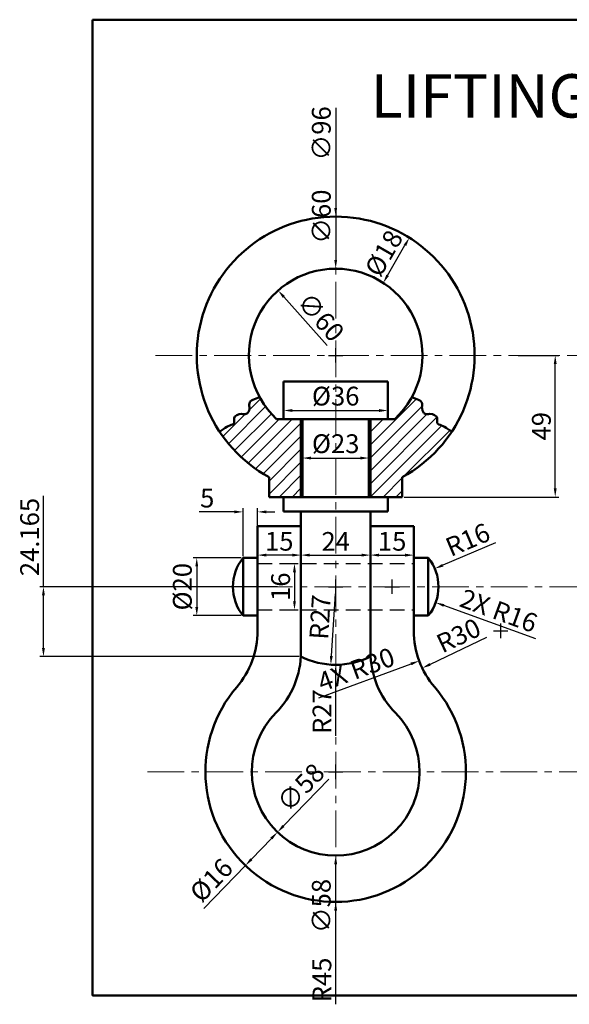
# Model space of a CAD drawing. Units: millimetres. Extents: x 309 to 670, y -17 to 339.
# Tile 1 of 2: x 309 to 498, y -2 to 339. Entities that reach past the tile are written whole.
import ezdxf

# ---------------------------------------------------------------- set-up
doc = ezdxf.new("R2010")
doc.units = ezdxf.units.MM
doc.header["$LTSCALE"] = 0.4
doc.linetypes.add('CENTER', pattern=[50.8, 31.75, -6.35, 6.35, -6.35])
doc.linetypes.add('DASHED', pattern=[19.05, 12.7, -6.35])
for name, color, linetype, lineweight in [('M-CNTR', 1, 'CENTER', 18), ('M-DIMS', 2, 'Continuous', 25), ('M-HATC', 8, 'Continuous', 18), ('M-HIDN', 3, 'DASHED', 25), ('M-OUTL', 7, 'Continuous', 50), ('M-TEXT', 7, 'Continuous', 25), ('M-TTLB', 7, 'Continuous', 50)]:
    doc.layers.add(name, color=color, linetype=linetype, lineweight=lineweight)
doc.styles.get("Standard").update_dxf_attribs({"font": 'arial.ttf'})
doc.dimstyles.new('ISO-25', dxfattribs={"dimtxt": 6.5, "dimasz": 3, "dimexe": 1.25, "dimexo": 0.625, "dimtad": 1, "dimdec": 0, "dimtxsty": 'Standard', "dimcen": 2.5, "dimadec": 0, "dimazin": 0, "dimtfac": 1, "dimtdec": 0, "dimtofl": 0, "dimtmove": 0, "dimatfit": 3, "dimfxl": 1, "dimarcsym": 0})

# ---------------------------------------------------------------- blocks, each defined once
blk = doc.blocks.new('*D13')
at = {"layer": 'Defpoints', "color": 0, "ltscale": 0.4, "transparency": 16777216}
for p in [(437.86, 99.54), (397.62, 57.77)]:
    blk.add_point(p, dxfattribs=at)
at = {"layer": 'M-DIMS', "color": 0, "lineweight": -2, "ltscale": 0.4, "transparency": 16777216}
blk.add_line((415.34, 76.16), (399.7, 59.93), dxfattribs=at)
at = {"layer": 'M-DIMS', "color": 0, "ltscale": 0.4, "transparency": 16777216}
blk.add_solid([(399.34, 60.27), (400.07, 59.58), (397.62, 57.77)], dxfattribs=at)
at = {"layer": 'M-DIMS', "color": 0, "ltscale": 0.4, "transparency": 16777216, "insert": (406.25, 72.67), "char_height": 6.5, "attachment_point": 5, "rotation": 46.0797}
blk.add_mtext('∅58', dxfattribs=at)
blk = doc.blocks.new('*D14')
at = {"layer": 'Defpoints', "color": 0, "ltscale": 0.4, "transparency": 16777216}
for p in [(397.62, 57.77), (386.53, 46.24), (386.53, 46.24)]:
    blk.add_point(p, dxfattribs=at)
at = {"layer": 'M-DIMS', "color": 0, "lineweight": -2, "ltscale": 0.4, "transparency": 16777216}
for p, q in [((397.17, 58.2), (396.72, 58.63)), ((395.54, 55.61), (388.61, 48.4)), ((386.53, 46.24), (372.22, 31.38)), ((386.08, 46.68), (385.63, 47.11))]:
    blk.add_line(p, q, dxfattribs=at)
at = {"layer": 'M-DIMS', "color": 0, "ltscale": 0.4, "transparency": 16777216}
for points in [[(395.18, 55.95), (395.9, 55.26), (397.62, 57.77)], [(388.25, 48.75), (388.97, 48.06), (386.53, 46.24)]]:
    blk.add_solid(points, dxfattribs=at)
at = {"layer": 'M-DIMS', "color": 0, "ltscale": 0.4, "transparency": 16777216, "insert": (375.36, 40.59), "char_height": 6.5, "attachment_point": 5, "rotation": 46.0797}
blk.add_mtext('%%C16', dxfattribs=at)
blk = doc.blocks.new('*D15')
at = {"layer": 'Defpoints', "color": 0, "ltscale": 0.4, "transparency": 16777216}
for p in [(390.74, 168.54), (385.74, 152.66), (390.74, 152.66)]:
    blk.add_point(p, dxfattribs=at)
at = {"layer": 'M-DIMS', "color": 0, "lineweight": -2, "ltscale": 0.4, "transparency": 16777216}
for p, q in [((382.74, 168.54), (370.57, 168.54)), ((385.74, 153.28), (385.74, 169.79)), ((390.74, 153.28), (390.74, 169.79)), ((393.74, 168.54), (396.74, 168.54))]:
    blk.add_line(p, q, dxfattribs=at)
at = {"layer": 'M-DIMS', "color": 0, "ltscale": 0.4, "transparency": 16777216}
for points in [[(382.74, 169.04), (382.74, 168.04), (385.74, 168.54)], [(393.74, 169.04), (393.74, 168.04), (390.74, 168.54)]]:
    blk.add_solid(points, dxfattribs=at)
at = {"layer": 'M-DIMS', "color": 0, "ltscale": 0.4, "transparency": 16777216, "insert": (373.35, 172.47), "char_height": 6.5, "attachment_point": 5}
blk.add_mtext('5', dxfattribs=at)
blk = doc.blocks.new('*D16')
at = {"layer": 'Defpoints', "color": 0, "ltscale": 0.4, "transparency": 16777216}
for p in [(429.74, 157.6), (444.74, 157.6), (444.74, 153.59)]:
    blk.add_point(p, dxfattribs=at)
at = {"layer": 'M-DIMS', "color": 0, "lineweight": -2, "ltscale": 0.4, "transparency": 16777216}
for p, q in [((429.74, 156.97), (429.74, 152.34)), ((444.74, 156.97), (444.74, 152.34)), ((432.74, 153.59), (441.74, 153.59))]:
    blk.add_line(p, q, dxfattribs=at)
at = {"layer": 'M-DIMS', "color": 0, "ltscale": 0.4, "transparency": 16777216}
for points in [[(432.74, 154.09), (432.74, 153.09), (429.74, 153.59)], [(441.74, 154.09), (441.74, 153.09), (444.74, 153.59)]]:
    blk.add_solid(points, dxfattribs=at)
at = {"layer": 'M-DIMS', "color": 0, "ltscale": 0.4, "transparency": 16777216, "insert": (437.24, 157.54), "char_height": 6.5, "attachment_point": 5}
blk.add_mtext('15', dxfattribs=at)
blk = doc.blocks.new('*D17')
at = {"layer": 'Defpoints', "color": 0, "ltscale": 0.4, "transparency": 16777216}
for p in [(405.74, 156.29), (429.74, 154.66), (429.74, 153.59)]:
    blk.add_point(p, dxfattribs=at)
at = {"layer": 'M-DIMS', "color": 0, "lineweight": -2, "ltscale": 0.4, "transparency": 16777216}
for p, q in [((405.74, 155.67), (405.74, 152.34)), ((408.74, 153.59), (426.74, 153.59)), ((429.74, 154.03), (429.74, 152.34))]:
    blk.add_line(p, q, dxfattribs=at)
at = {"layer": 'M-DIMS', "color": 0, "ltscale": 0.4, "transparency": 16777216}
for points in [[(408.74, 154.09), (408.74, 153.09), (405.74, 153.59)], [(426.74, 154.09), (426.74, 153.09), (429.74, 153.59)]]:
    blk.add_solid(points, dxfattribs=at)
at = {"layer": 'M-DIMS', "color": 0, "ltscale": 0.4, "transparency": 16777216, "insert": (417.74, 157.48), "char_height": 6.5, "attachment_point": 5}
blk.add_mtext('24', dxfattribs=at)
blk = doc.blocks.new('*D18')
at = {"layer": 'Defpoints', "color": 0, "ltscale": 0.4, "transparency": 16777216}
for p in [(390.74, 153.59), (390.74, 153.59), (405.74, 153.59)]:
    blk.add_point(p, dxfattribs=at)
at = {"layer": 'M-DIMS', "color": 0, "lineweight": -2, "ltscale": 0.4, "transparency": 16777216}
for p, q in [((390.74, 154.22), (390.74, 154.84)), ((402.74, 153.59), (393.74, 153.59)), ((405.74, 154.22), (405.74, 154.84))]:
    blk.add_line(p, q, dxfattribs=at)
at = {"layer": 'M-DIMS', "color": 0, "ltscale": 0.4, "transparency": 16777216}
for points in [[(393.74, 154.09), (393.74, 153.09), (390.74, 153.59)], [(402.74, 154.09), (402.74, 153.09), (405.74, 153.59)]]:
    blk.add_solid(points, dxfattribs=at)
at = {"layer": 'M-DIMS', "color": 0, "ltscale": 0.4, "transparency": 16777216, "insert": (398.24, 157.54), "char_height": 6.5, "attachment_point": 5}
blk.add_mtext('15', dxfattribs=at)
blk = doc.blocks.new('*D19')
at = {"layer": 'Defpoints', "color": 0, "ltscale": 0.4, "transparency": 16777216}
for p in [(399.65, 150.66), (399.65, 134.66), (403.5, 134.66)]:
    blk.add_point(p, dxfattribs=at)
at = {"layer": 'M-DIMS', "color": 0, "lineweight": -2, "ltscale": 0.4, "transparency": 16777216}
for p, q in [((400.28, 150.66), (404.75, 150.66)), ((403.5, 147.66), (403.5, 137.66)), ((400.28, 134.66), (404.75, 134.66))]:
    blk.add_line(p, q, dxfattribs=at)
at = {"layer": 'M-DIMS', "color": 0, "ltscale": 0.4, "transparency": 16777216}
for points in [[(403, 147.66), (404, 147.66), (403.5, 150.66)], [(403, 137.66), (404, 137.66), (403.5, 134.66)]]:
    blk.add_solid(points, dxfattribs=at)
at = {"layer": 'M-DIMS', "color": 0, "ltscale": 0.4, "transparency": 16777216, "insert": (399.55, 142.66), "char_height": 6.5, "attachment_point": 5, "rotation": 90}
blk.add_mtext('16', dxfattribs=at)
blk = doc.blocks.new('*D20')
at = {"layer": 'Defpoints', "color": 0, "ltscale": 0.4, "transparency": 16777216}
for p in [(385.74, 152.66), (369.74, 132.66), (385.74, 132.66)]:
    blk.add_point(p, dxfattribs=at)
at = {"layer": 'M-DIMS', "color": 0, "lineweight": -2, "ltscale": 0.4, "transparency": 16777216}
for p, q in [((385.11, 152.66), (368.49, 152.66)), ((369.74, 149.66), (369.74, 135.66)), ((385.11, 132.66), (368.49, 132.66))]:
    blk.add_line(p, q, dxfattribs=at)
at = {"layer": 'M-DIMS', "color": 0, "ltscale": 0.4, "transparency": 16777216}
for points in [[(369.24, 149.66), (370.24, 149.66), (369.74, 152.66)], [(369.24, 135.66), (370.24, 135.66), (369.74, 132.66)]]:
    blk.add_solid(points, dxfattribs=at)
at = {"layer": 'M-DIMS', "color": 0, "ltscale": 0.4, "transparency": 16777216, "insert": (365.61, 142.66), "char_height": 6.5, "attachment_point": 5, "rotation": 90}
blk.add_mtext('%%C20', dxfattribs=at)
blk = doc.blocks.new('*D21')
at = {"layer": 'Defpoints', "color": 0, "ltscale": 0.4, "transparency": 16777216}
for p in [(451.98, 148.91), (437.25, 142.66)]:
    blk.add_point(p, dxfattribs=at)
at = {"layer": 'M-DIMS', "color": 0, "lineweight": -2, "ltscale": 0.4, "transparency": 16777216}
for p, q in [((472.95, 157.8), (454.74, 150.08)), ((437.25, 140.16), (437.25, 145.16)), ((434.75, 142.66), (439.75, 142.66))]:
    blk.add_line(p, q, dxfattribs=at)
at = {"layer": 'M-DIMS', "color": 0, "ltscale": 0.4, "transparency": 16777216}
blk.add_solid([(454.54, 150.54), (454.94, 149.62), (451.98, 148.91)], dxfattribs=at)
at = {"layer": 'M-DIMS', "color": 0, "ltscale": 0.4, "transparency": 16777216, "insert": (463.68, 158.16), "char_height": 6.5, "attachment_point": 5, "rotation": 22.9948}
blk.add_mtext('R16', dxfattribs=at)
blk = doc.blocks.new('*D22')
at = {"layer": 'Defpoints', "color": 0, "ltscale": 0.4, "transparency": 16777216}
for p in [(417.74, 142.66), (416.04, 115.71)]:
    blk.add_point(p, dxfattribs=at)
at = {"layer": 'M-DIMS', "color": 0, "lineweight": -2, "ltscale": 0.4, "transparency": 16777216}
blk.add_line((417.59, 140.23), (416.23, 118.7), dxfattribs=at)
at = {"layer": 'M-DIMS', "color": 0, "ltscale": 0.4, "transparency": 16777216}
blk.add_solid([(415.73, 118.73), (416.73, 118.67), (416.04, 115.71)], dxfattribs=at)
at = {"layer": 'M-DIMS', "color": 0, "ltscale": 0.4, "transparency": 16777216, "insert": (413.18, 132.1), "char_height": 6.5, "attachment_point": 5, "rotation": 86.3929}
blk.add_mtext('R27', dxfattribs=at)
blk = doc.blocks.new('*D23')
at = {"layer": 'Defpoints', "color": 0, "ltscale": 0.4, "transparency": 16777216}
for p in [(474.74, 127.4), (447.65, 114.52)]:
    blk.add_point(p, dxfattribs=at)
at = {"layer": 'M-DIMS', "color": 0, "lineweight": -2, "ltscale": 0.4, "transparency": 16777216}
blk.add_line((469.82, 125.06), (450.35, 115.81), dxfattribs=at)
at = {"layer": 'M-DIMS', "color": 0, "ltscale": 0.4, "transparency": 16777216}
blk.add_solid([(450.14, 116.26), (450.57, 115.36), (447.65, 114.52)], dxfattribs=at)
at = {"layer": 'M-DIMS', "color": 0, "ltscale": 0.4, "transparency": 16777216, "insert": (460.55, 125.03), "char_height": 6.5, "attachment_point": 5, "rotation": 25.4233}
blk.add_mtext('R30', dxfattribs=at)
blk = doc.blocks.new('*D24')
at = {"layer": 'Defpoints', "color": 0, "ltscale": 0.4, "transparency": 16777216}
for p in [(397.85, 245.11), (437.63, 200.2)]:
    blk.add_point(p, dxfattribs=at)
at = {"layer": 'M-DIMS', "color": 0, "lineweight": -2, "ltscale": 0.4, "transparency": 16777216}
blk.add_line((414.76, 226.03), (399.84, 242.87), dxfattribs=at)
at = {"layer": 'M-DIMS', "color": 0, "ltscale": 0.4, "transparency": 16777216}
blk.add_solid([(400.21, 243.2), (399.46, 242.53), (397.85, 245.11)], dxfattribs=at)
at = {"layer": 'M-DIMS', "color": 0, "ltscale": 0.4, "transparency": 16777216, "insert": (412, 235.35), "char_height": 6.5, "attachment_point": 5, "rotation": 311.5346}
blk.add_mtext('∅60', dxfattribs=at)
blk = doc.blocks.new('*D25')
at = {"layer": 'Defpoints', "color": 0, "ltscale": 0.4, "transparency": 16777216}
for p in [(439.85, 265.26), (443.18, 263.34), (430.83, 249.65)]:
    blk.add_point(p, dxfattribs=at)
at = {"layer": 'M-DIMS', "color": 0, "lineweight": -2, "ltscale": 0.4, "transparency": 16777216}
for p, q in [((440.39, 264.95), (444.26, 262.71)), ((435.66, 250.32), (441.68, 260.74)), ((431.38, 249.33), (435.25, 247.1))]:
    blk.add_line(p, q, dxfattribs=at)
at = {"layer": 'M-DIMS', "color": 0, "ltscale": 0.4, "transparency": 16777216}
for points in [[(441.25, 260.99), (442.11, 260.49), (443.18, 263.34)], [(435.23, 250.57), (436.1, 250.07), (434.16, 247.72)]]:
    blk.add_solid(points, dxfattribs=at)
at = {"layer": 'M-DIMS', "color": 0, "ltscale": 0.4, "transparency": 16777216, "insert": (435.1, 257.59), "char_height": 6.5, "attachment_point": 5, "rotation": 60}
blk.add_mtext('%%C18', dxfattribs=at)
blk = doc.blocks.new('*D26')
at = {"layer": 'Defpoints', "color": 0, "ltscale": 0.4, "transparency": 16777216}
for p in [(480.2, 222.66), (493.58, 222.66), (440.74, 173.66)]:
    blk.add_point(p, dxfattribs=at)
at = {"layer": 'M-DIMS', "color": 0, "lineweight": -2, "ltscale": 0.4, "transparency": 16777216}
for p, q in [((480.83, 222.66), (494.83, 222.66)), ((493.58, 176.66), (493.58, 219.66)), ((441.36, 173.66), (494.83, 173.66))]:
    blk.add_line(p, q, dxfattribs=at)
at = {"layer": 'M-DIMS', "color": 0, "ltscale": 0.4, "transparency": 16777216}
for points in [[(493.08, 219.66), (494.08, 219.66), (493.58, 222.66)], [(493.08, 176.66), (494.08, 176.66), (493.58, 173.66)]]:
    blk.add_solid(points, dxfattribs=at)
at = {"layer": 'M-DIMS', "color": 0, "ltscale": 0.4, "transparency": 16777216, "insert": (489.64, 198.16), "char_height": 6.5, "attachment_point": 5, "rotation": 90}
blk.add_mtext('49', dxfattribs=at)
blk = doc.blocks.new('*D27')
at = {"layer": 'Defpoints', "color": 0, "ltscale": 0.4, "transparency": 16777216}
for p in [(399.74, 207.16), (435.74, 207.16), (435.74, 203.6)]:
    blk.add_point(p, dxfattribs=at)
at = {"layer": 'M-DIMS', "color": 0, "lineweight": -2, "ltscale": 0.4, "transparency": 16777216}
for p, q in [((399.74, 206.53), (399.74, 202.35)), ((435.74, 206.53), (435.74, 202.35)), ((402.74, 203.6), (432.74, 203.6))]:
    blk.add_line(p, q, dxfattribs=at)
at = {"layer": 'M-DIMS', "color": 0, "ltscale": 0.4, "transparency": 16777216}
for points in [[(402.74, 204.1), (402.74, 203.1), (399.74, 203.6)], [(432.74, 204.1), (432.74, 203.1), (435.74, 203.6)]]:
    blk.add_solid(points, dxfattribs=at)
at = {"layer": 'M-DIMS', "color": 0, "ltscale": 0.4, "transparency": 16777216, "insert": (417.74, 207.73), "char_height": 6.5, "attachment_point": 5}
blk.add_mtext('%%C36', dxfattribs=at)
blk = doc.blocks.new('*D28')
at = {"layer": 'Defpoints', "color": 0, "ltscale": 0.4, "transparency": 16777216}
for p in [(406.24, 187.16), (429.24, 187.16), (429.24, 187.16)]:
    blk.add_point(p, dxfattribs=at)
at = {"layer": 'M-DIMS', "color": 0, "lineweight": -2, "ltscale": 0.4, "transparency": 16777216}
for p, q in [((406.24, 187.78), (406.24, 188.41)), ((429.24, 187.78), (429.24, 188.41)), ((409.24, 187.16), (426.24, 187.16))]:
    blk.add_line(p, q, dxfattribs=at)
at = {"layer": 'M-DIMS', "color": 0, "ltscale": 0.4, "transparency": 16777216}
for points in [[(409.24, 187.66), (409.24, 186.66), (406.24, 187.16)], [(426.24, 187.66), (426.24, 186.66), (429.24, 187.16)]]:
    blk.add_solid(points, dxfattribs=at)
at = {"layer": 'M-DIMS', "color": 0, "ltscale": 0.4, "transparency": 16777216, "insert": (417.74, 191.28), "char_height": 6.5, "attachment_point": 5}
blk.add_mtext('%%C23', dxfattribs=at)
blk = doc.blocks.new('*D30')
at = {"layer": 'Defpoints', "color": 0, "ltscale": 0.4, "transparency": 16777216}
for p in [(316.78, 142.66), (398.23, 142.66), (405.7, 118.49)]:
    blk.add_point(p, dxfattribs=at)
at = {"layer": 'M-DIMS', "color": 0, "lineweight": -2, "ltscale": 0.4, "transparency": 16777216}
for p, q in [((316.78, 142.66), (316.78, 174.05)), ((397.6, 142.66), (315.53, 142.66)), ((316.78, 121.49), (316.78, 139.66)), ((405.07, 118.49), (315.53, 118.49))]:
    blk.add_line(p, q, dxfattribs=at)
at = {"layer": 'M-DIMS', "color": 0, "ltscale": 0.4, "transparency": 16777216}
for points in [[(316.28, 139.66), (317.28, 139.66), (316.78, 142.66)], [(316.28, 121.49), (317.28, 121.49), (316.78, 118.49)]]:
    blk.add_solid(points, dxfattribs=at)
at = {"layer": 'M-DIMS', "color": 0, "ltscale": 0.4, "transparency": 16777216, "insert": (312.84, 159.85), "char_height": 6.5, "attachment_point": 5, "rotation": 90}
blk.add_mtext('24.165', dxfattribs=at)
blk = doc.blocks.new('*D33')
at = {"layer": 'Defpoints', "color": 0, "ltscale": 0.4, "transparency": 16777216}
for p in [(417.74, 270.66), (417.74, 174.66)]:
    blk.add_point(p, dxfattribs=at)
at = {"layer": 'M-DIMS', "color": 0, "lineweight": -2, "ltscale": 0.4, "transparency": 16777216}
for p, q in [((417.74, 308.27), (417.74, 273.66)), ((417.74, 220.16), (417.74, 225.16)), ((415.24, 222.66), (420.24, 222.66))]:
    blk.add_line(p, q, dxfattribs=at)
at = {"layer": 'M-DIMS', "color": 0, "ltscale": 0.4, "transparency": 16777216}
blk.add_solid([(417.24, 273.66), (418.24, 273.66), (417.74, 270.66)], dxfattribs=at)
at = {"layer": 'M-DIMS', "color": 0, "ltscale": 0.4, "transparency": 16777216, "insert": (413.61, 299.46), "char_height": 6.5, "attachment_point": 5, "rotation": 90}
blk.add_mtext('∅96', dxfattribs=at)
blk = doc.blocks.new('*D34')
at = {"layer": 'Defpoints', "color": 0, "ltscale": 0.4, "transparency": 16777216}
for p in [(417.74, 252.66), (417.74, 192.66)]:
    blk.add_point(p, dxfattribs=at)
at = {"layer": 'M-DIMS', "color": 0, "lineweight": -2, "ltscale": 0.4, "transparency": 16777216}
for p, q in [((417.74, 279.46), (417.74, 255.66)), ((417.74, 220.16), (417.74, 225.16)), ((415.24, 222.66), (420.24, 222.66))]:
    blk.add_line(p, q, dxfattribs=at)
at = {"layer": 'M-DIMS', "color": 0, "ltscale": 0.4, "transparency": 16777216}
blk.add_solid([(417.24, 255.66), (418.24, 255.66), (417.74, 252.66)], dxfattribs=at)
at = {"layer": 'M-DIMS', "color": 0, "ltscale": 0.4, "transparency": 16777216, "insert": (413.61, 270.66), "char_height": 6.5, "attachment_point": 5, "rotation": 90}
blk.add_mtext('∅60', dxfattribs=at)
blk = doc.blocks.new('*D35')
at = {"layer": 'Defpoints', "color": 0, "ltscale": 0.4, "transparency": 16777216}
for p in [(417.74, 107.66), (417.74, 49.66)]:
    blk.add_point(p, dxfattribs=at)
at = {"layer": 'M-DIMS', "color": 0, "lineweight": -2, "ltscale": 0.4, "transparency": 16777216}
for p, q in [((415.24, 78.66), (420.24, 78.66)), ((417.74, 76.16), (417.74, 81.16)), ((417.74, 23.43), (417.74, 46.66))]:
    blk.add_line(p, q, dxfattribs=at)
at = {"layer": 'M-DIMS', "color": 0, "ltscale": 0.4, "transparency": 16777216}
blk.add_solid([(417.24, 46.66), (418.24, 46.66), (417.74, 49.66)], dxfattribs=at)
at = {"layer": 'M-DIMS', "color": 0, "ltscale": 0.4, "transparency": 16777216, "insert": (413.61, 32.26), "char_height": 6.5, "attachment_point": 5, "rotation": 90}
blk.add_mtext('∅58', dxfattribs=at)
blk = doc.blocks.new('*D36')
at = {"layer": 'Defpoints', "color": 0, "ltscale": 0.4, "transparency": 16777216}
for p in [(417.74, 78.66), (417.74, 33.66)]:
    blk.add_point(p, dxfattribs=at)
at = {"layer": 'M-DIMS', "color": 0, "lineweight": -2, "ltscale": 0.4, "transparency": 16777216}
for p, q in [((415.24, 78.66), (420.24, 78.66)), ((417.74, 76.16), (417.74, 81.16)), ((417.74, -1.76), (417.74, 30.66))]:
    blk.add_line(p, q, dxfattribs=at)
at = {"layer": 'M-DIMS', "color": 0, "ltscale": 0.4, "transparency": 16777216}
blk.add_solid([(417.24, 30.66), (418.24, 30.66), (417.74, 33.66)], dxfattribs=at)
at = {"layer": 'M-DIMS', "color": 0, "ltscale": 0.4, "transparency": 16777216, "insert": (413.81, 6.66), "char_height": 6.5, "attachment_point": 5, "rotation": 90}
blk.add_mtext('R45', dxfattribs=at)
blk = doc.blocks.new('*D37')
at = {"layer": 'Defpoints', "color": 0, "ltscale": 0.4, "transparency": 16777216}
for p in [(474.74, 127.4), (446.6, 117.01)]:
    blk.add_point(p, dxfattribs=at)
at = {"layer": 'M-DIMS', "color": 0, "lineweight": -2, "ltscale": 0.4, "transparency": 16777216}
for p, q in [((474.74, 124.9), (474.74, 129.9)), ((472.24, 127.4), (477.24, 127.4)), ((411.9, 104.19), (443.78, 115.97))]:
    blk.add_line(p, q, dxfattribs=at)
at = {"layer": 'M-DIMS', "color": 0, "ltscale": 0.4, "transparency": 16777216}
blk.add_solid([(443.61, 116.44), (443.96, 115.5), (446.6, 117.01)], dxfattribs=at)
at = {"layer": 'M-DIMS', "color": 0, "ltscale": 0.4, "transparency": 16777216, "insert": (425.07, 113.26), "char_height": 6.5, "attachment_point": 5, "rotation": 20.269}
blk.add_mtext('4X R30', dxfattribs=at)
blk = doc.blocks.new('*D38')
at = {"layer": 'Defpoints', "color": 0, "ltscale": 0.4, "transparency": 16777216}
for p in [(417.74, 142.66), (417.74, 115.66)]:
    blk.add_point(p, dxfattribs=at)
at = {"layer": 'M-DIMS', "color": 0, "lineweight": -2, "ltscale": 0.4, "transparency": 16777216}
for p, q in [((417.74, 140.16), (417.74, 145.16)), ((415.24, 142.66), (420.24, 142.66)), ((417.74, 91.06), (417.74, 112.66))]:
    blk.add_line(p, q, dxfattribs=at)
at = {"layer": 'M-DIMS', "color": 0, "ltscale": 0.4, "transparency": 16777216}
blk.add_solid([(417.24, 112.66), (418.24, 112.66), (417.74, 115.66)], dxfattribs=at)
at = {"layer": 'M-DIMS', "color": 0, "ltscale": 0.4, "transparency": 16777216, "insert": (413.85, 99.46), "char_height": 6.5, "attachment_point": 5, "rotation": 90}
blk.add_mtext('R27', dxfattribs=at)
blk = doc.blocks.new('*D39')
at = {"layer": 'Defpoints', "color": 0, "ltscale": 0.4, "transparency": 16777216}
for p in [(437.25, 142.66), (452.29, 137.19)]:
    blk.add_point(p, dxfattribs=at)
at = {"layer": 'M-DIMS', "color": 0, "lineweight": -2, "ltscale": 0.4, "transparency": 16777216}
for p, q in [((437.25, 140.16), (437.25, 145.16)), ((434.75, 142.66), (439.75, 142.66)), ((486.93, 124.6), (455.11, 136.17))]:
    blk.add_line(p, q, dxfattribs=at)
at = {"layer": 'M-DIMS', "color": 0, "ltscale": 0.4, "transparency": 16777216}
blk.add_solid([(455.28, 136.64), (454.94, 135.7), (452.29, 137.19)], dxfattribs=at)
at = {"layer": 'M-DIMS', "color": 0, "ltscale": 0.4, "transparency": 16777216, "insert": (473.77, 133.58), "char_height": 6.5, "attachment_point": 5, "rotation": 340.0289}
blk.add_mtext('2X R16', dxfattribs=at)

msp = doc.modelspace()

# ---------------------------------------------------------------- hatches: boundary and pattern name
at = {"layer": 'M-HATC', "ltscale": 0.4}
h = msp.add_hatch(dxfattribs=at)
h.set_pattern_fill('ANSI31', color=256)
edge = h.paths.add_edge_path()
edge.add_line((405.74, 200.6555), (399.74, 200.6555))
edge.add_line((399.74, 200.6555), (397.3439, 200.6555))
edge.add_arc((417.74, 222.6555), 30, 209.008501, 227.166572, ccw=False)
edge.add_spline(control_points=[(391.5036, 208.1073), (389.826, 207.6499), (387.4257, 206.9953), (388.1722, 204.1549), (387.1237, 201.9948), (384.8006, 202.7074), (382.0626, 201.6056), (383.111, 199.0273), (380.8035, 198.4287), (379.327, 197.3703), (378.1433, 196.602), (377.6394, 196.2748)], knot_values=[0, 0, 0, 0, 4.1475584, 5.93440089, 8.06363155, 9.72120684, 12.66639102, 14.31534035, 15.96407937, 18.3684954, 20.15124589, 20.15124589, 20.15124589, 20.15124589], degree=3, periodic=0)
edge.add_arc((417.74, 222.6555), 48, 213.339412, 241.36901)
edge.add_line((394.74, 180.5248), (394.74, 173.6555))
edge.add_line((394.74, 173.6555), (399.74, 173.6555))
edge.add_line((399.74, 173.6555), (405.74, 173.6555))
edge.add_line((405.74, 173.6555), (405.74, 200.6555))
edge = h.paths.add_edge_path()
edge.add_spline(control_points=[(457.8406, 196.2748), (457.3367, 196.602), (456.153, 197.3703), (454.6765, 198.4287), (452.369, 199.0273), (453.4174, 201.6056), (450.6794, 202.7074), (448.3563, 201.9948), (447.3078, 204.1549), (448.0543, 206.9953), (445.654, 207.6499), (443.9764, 208.1073)], knot_values=[0, 0, 0, 0, 1.78275049, 4.18716652, 5.83590555, 7.48485488, 10.43003905, 12.08761434, 14.216845, 16.00368749, 20.15124589, 20.15124589, 20.15124589, 20.15124589], degree=3, periodic=0)
edge.add_arc((417.74, 222.6555), 30, 312.833428, 330.991499, ccw=False)
edge.add_line((438.1361, 200.6555), (435.74, 200.6555))
edge.add_line((435.74, 200.6555), (429.74, 200.6555))
edge.add_line((429.74, 200.6555), (429.74, 173.6555))
edge.add_line((429.74, 173.6555), (435.74, 173.6555))
edge.add_line((435.74, 173.6555), (440.74, 173.6555))
edge.add_line((440.74, 173.6555), (440.74, 180.5248))
edge.add_arc((417.74, 222.6555), 48, 298.63099, 326.660588)

# ---------------------------------------------------------------- linework, layer by layer
at = {"layer": 'M-CNTR'}
for p, q in [((417.74, 288.7904), (417.74, 28.1721)), ((355.4751, 222.6555), (604.9301, 222.6555)), ((369.74, 142.6555), (604.9301, 142.6555)), ((352.7304, 78.6555), (604.9301, 78.6555))]:
    msp.add_line(p, q, dxfattribs=at)
at = {"layer": 'M-HIDN'}
for p, q in [((390.74, 150.6555), (444.74, 150.6555)), ((390.74, 134.6555), (444.74, 134.6555))]:
    msp.add_line(p, q, dxfattribs=at)
at = {"layer": 'M-OUTL', "ltscale": 0.4}
for p, q in [((435.74, 213.6555), (399.74, 213.6555)), ((399.74, 213.6555), (399.74, 200.6555)), ((399.74, 200.6555), (399.74, 213.6555)), ((435.74, 200.6555), (435.74, 213.6555)), ((399.74, 200.6555), (397.3439, 200.6555)), ((399.74, 200.6555), (435.74, 200.6555)), ((405.74, 200.6555), (405.74, 173.6555)), ((406.24, 200.6555), (406.24, 173.6555)), ((429.24, 200.6555), (429.24, 173.6555)), ((429.74, 200.6555), (429.74, 173.6555)), ((435.74, 200.6555), (438.1361, 200.6555)), ((394.74, 173.6555), (394.74, 180.5248)), ((440.74, 173.6555), (440.74, 180.5248)), ((399.74, 173.6555), (394.74, 173.6555)), ((435.74, 173.6555), (440.74, 173.6555))]:
    msp.add_line(p, q, dxfattribs=at)
at = {"layer": 'M-OUTL'}
for p, q in [((399.74, 173.6555), (435.74, 173.6555)), ((399.74, 173.6555), (399.74, 168.6555)), ((435.74, 173.6555), (435.74, 168.6555)), ((399.74, 168.6555), (435.74, 168.6555)), ((405.74, 168.6555), (405.74, 120.0922)), ((429.74, 168.6555), (429.74, 120.0922)), ((390.74, 163.6555), (390.74, 127.3997)), ((405.74, 163.6555), (390.74, 163.6555)), ((444.74, 163.6555), (429.74, 163.6555)), ((444.74, 163.6555), (444.74, 127.3997)), ((385.74, 152.6555), (385.74, 132.6555)), ((390.74, 152.6555), (385.74, 152.6555)), ((390.74, 132.6555), (390.74, 152.6555)), ((444.74, 152.6555), (444.74, 132.6555)), ((449.74, 152.6555), (444.74, 152.6555)), ((449.74, 132.6555), (449.74, 152.6555)), ((385.74, 132.6555), (390.74, 132.6555)), ((444.74, 132.6555), (449.74, 132.6555))]:
    msp.add_line(p, q, dxfattribs=at)
for centre, radius, start, end in [((417.74, 222.6555), 48, 298.63099, 241.36901), ((417.74, 222.6555), 30, 312.833428, 227.166572), ((360.74, 127.3997), 30, 319.464198, 0), ((474.74, 127.3997), 30, 180, 220.535802), ((375.74, 120.0922), 30, 315.386812, 360), ((459.74, 120.0922), 30, 180, 224.613188), ((417.74, 78.6555), 45, 139.464198, 40.535802), ((417.74, 78.6555), 29, 135.386812, 44.613188)]:
    msp.add_arc(centre, radius, start, end, dxfattribs=at)
at = {"layer": 'M-OUTL', "ltscale": 0.4}
for centre, radius, start, end in [((398.23, 142.6555), 16, 141.317813, 218.682187), ((437.25, 142.6555), 16, 321.317813, 38.682187), ((417.74, 142.6555), 27, 243.510734, 296.489266)]:
    msp.add_arc(centre, radius, start, end, dxfattribs=at)
for points in [[(391.5036, 208.1073), (389.826, 207.6499), (387.4257, 206.9953), (388.1722, 204.1549), (387.1237, 201.9948), (384.8006, 202.7074), (382.0626, 201.6056), (383.111, 199.0273), (380.8035, 198.4287), (379.327, 197.3703), (378.1433, 196.602), (377.6394, 196.2748)], [(443.9764, 208.1073), (445.654, 207.6499), (448.0543, 206.9953), (447.3078, 204.1549), (448.3563, 201.9948), (450.6794, 202.7074), (453.4174, 201.6056), (452.369, 199.0273), (454.6765, 198.4287), (456.153, 197.3703), (457.3367, 196.602), (457.8406, 196.2748)]]:
    msp.add_open_spline(points, degree=3, knots=[0, 0, 0, 0, 4.1475584, 5.93440089, 8.06363155, 9.72120684, 12.66639102, 14.31534035, 15.96407937, 18.3684954, 20.15124589, 20.15124589, 20.15124589, 20.15124589], dxfattribs=at)
at = {"layer": 'M-TTLB', "ltscale": 0.4}
msp.add_lwpolyline([(333.7348, 338.7612), (651.3692, 338.7612), (651.3692, 1.3112), (333.7348, 1.3112)], close=True, dxfattribs=at)

# ---------------------------------------------------------------- texts
at = {"layer": 'M-TEXT', "ltscale": 0.4, "insert": (429.8042, 319.9085), "char_height": 15, "attachment_point": 1}
msp.add_mtext_dynamic_manual_height_columns('LIFTING HOOK', width=169.632423, gutter_width=12.5, heights=[0], dxfattribs=at)

# ---------------------------------------------------------------- dimensions: what is measured, and where the dimension line sits
at = {"layer": 'M-DIMS', "ltscale": 0.4}
for p1, p2, override, picture, middle in [((417.74, 174.6555), (417.74, 270.6555), {"dimdec": 0, "dimlfac": 1, "dimrnd": 0, "dimzin": 0, "dimdsep": 46, "dimlunit": 2}, '*D33', (417.74, 299.4555)), ((417.74, 192.6555), (417.74, 252.6555), {"dimdec": 0, "dimlfac": 1, "dimrnd": 0, "dimzin": 0, "dimdsep": 46, "dimlunit": 2}, '*D34', (417.74, 270.6555)), ((437.6322, 200.1988), (397.8478, 245.1122), {"dimclrd": 0, "dimclre": 0, "dimclrt": 0}, '*D24', (408.9166, 232.6164)), ((417.74, 107.6555), (417.74, 49.6555), {"dimdec": 0, "dimlfac": 1, "dimrnd": 0, "dimzin": 0, "dimdsep": 46, "dimlunit": 2}, '*D35', (417.74, 32.2555)), ((437.8561, 99.5444), (397.6239, 57.7667), {"dimclrd": 0, "dimclre": 0, "dimclrt": 0}, '*D13', (409.2184, 69.8066))]:
    dim = msp.add_diameter_dim_2p(p1=p1, p2=p2, dimstyle='ISO-25', override=override, dxfattribs=at)
    dim.commit()
    dim.dimension.update_dxf_attribs({"geometry": picture, "text_midpoint": middle, "dimtype": 163})
for p1, p2, distance, picture, middle in [((430.8347, 249.6468), (439.8492, 265.2605), -3.8452, '*D25', (435.0992, 257.5938)), ((397.6239, 57.7667), (386.5254, 46.2418), 0, '*D14', (375.3587, 40.5936))]:
    dim = msp.add_aligned_dim(p1=p1, p2=p2, distance=distance, text='%%C<>', dimstyle='ISO-25', override={"dimclrd": 0, "dimclre": 0, "dimclrt": 0}, dxfattribs=at)
    dim.commit()
    dim.dimension.update_dxf_attribs({"geometry": picture, "text_midpoint": middle})
for base, p1, p2, override, picture, middle in [((493.5804, 222.6555), (440.74, 173.6555), (480.2026, 222.6555), {"dimclrd": 0, "dimclre": 0, "dimclrt": 0}, '*D26', (489.6367, 198.1555)), ((316.78475, 142.65551), (405.69719, 118.49003), (398.23, 142.65551), {"dimdec": 3, "dimlfac": 1, "dimrnd": 0, "dimzin": 0, "dimdsep": 46, "dimlunit": 2}, '*D30', (312.84103, 159.85248)), ((403.4977, 134.6555), (399.6546, 150.6555), (399.6546, 134.6555), {"dimclrd": 0, "dimclre": 0, "dimclrt": 0}, '*D19', (399.554, 142.6555))]:
    dim = msp.add_linear_dim(base=base, p1=p1, p2=p2, angle=90, dimstyle='ISO-25', override=override, dxfattribs=at)
    dim.commit()
    dim.dimension.update_dxf_attribs({"geometry": picture, "text_midpoint": middle})
for base, p1, p2, picture, middle in [((435.74, 203.6016), (399.74, 207.1555), (435.74, 207.1555), '*D27', (417.74, 207.7271)), ((429.24, 187.1555), (406.24, 187.1555), (429.24, 187.1555), '*D28', (417.74, 191.281))]:
    dim = msp.add_linear_dim(base=base, p1=p1, p2=p2, text='%%C<>', dimstyle='ISO-25', override={"dimclrd": 0, "dimclre": 0, "dimclrt": 0}, dxfattribs=at)
    dim.commit()
    dim.dimension.update_dxf_attribs({"geometry": picture, "text_midpoint": middle})
dim = msp.add_linear_dim(base=(390.74, 168.5382), p1=(385.74, 152.6555), p2=(390.74, 152.6555), dimstyle='ISO-25', override={"dimclrd": 0, "dimclre": 0, "dimclrt": 0}, dxfattribs=at)
dim.commit()
dim.dimension.update_dxf_attribs({"geometry": '*D15', "text_midpoint": (373.3472, 168.5382), "dimtype": 160})
dim = msp.add_radius_dim(center=(437.25, 142.6555), mpoint=(451.9786, 148.9059), dimstyle='ISO-25', override={"dimclrd": 0, "dimclre": 0, "dimclrt": 0}, dxfattribs=at)
dim.commit()
dim.dimension.update_dxf_attribs({"geometry": '*D21', "text_midpoint": (463.6834, 158.1571)})
for base, p1, p2, picture, middle in [((390.74, 153.5917), (405.74, 153.5917), (390.74, 153.5917), '*D18', (398.24, 157.5355)), ((429.74, 153.5917), (405.74, 156.2907), (429.74, 154.6567), '*D17', (417.74, 157.4801)), ((444.74, 153.5917), (429.74, 157.5967), (444.74, 157.5967), '*D16', (437.24, 157.5355))]:
    dim = msp.add_linear_dim(base=base, p1=p1, p2=p2, dimstyle='ISO-25', override={"dimclrd": 0, "dimclre": 0, "dimclrt": 0}, dxfattribs=at)
    dim.commit()
    dim.dimension.update_dxf_attribs({"geometry": picture, "text_midpoint": middle})
dim = msp.add_linear_dim(base=(369.74, 132.6555), p1=(385.74, 152.6555), p2=(385.74, 132.6555), angle=90, text='%%C<>', dimstyle='ISO-25', override={"dimclrd": 0, "dimclre": 0, "dimclrt": 0}, dxfattribs=at)
dim.commit()
dim.dimension.update_dxf_attribs({"geometry": '*D20', "text_midpoint": (365.6145, 142.6555)})
for center, mpoint, override, picture, middle in [((417.74, 142.6555), (417.74, 115.6555), {"dimdec": 0, "dimlfac": 1, "dimrnd": 0, "dimzin": 0, "dimdsep": 46, "dimlunit": 2}, '*D38', (417.74, 99.4555)), ((417.74, 142.6555), (416.0413, 115.709), {"dimclrd": 0, "dimclre": 0, "dimclrt": 0}, '*D22', (417.0595, 131.8599)), ((474.74, 127.3997), (447.6452, 114.5207), {"dimclrd": 0, "dimclre": 0, "dimclrt": 0}, '*D23', (462.2487, 121.4622)), ((417.74, 78.6555), (417.74, 33.6555), {"dimdec": 0, "dimlfac": 1, "dimrnd": 0, "dimzin": 0, "dimdsep": 46, "dimlunit": 2}, '*D36', (417.74, 6.6555))]:
    dim = msp.add_radius_dim(center=center, mpoint=mpoint, dimstyle='ISO-25', override=override, dxfattribs=at)
    dim.commit()
    dim.dimension.update_dxf_attribs({"geometry": picture, "text_midpoint": middle, "dimtype": 164})
for center, mpoint, text, picture, middle in [((437.25, 142.6555), (452.2878, 137.1908), '2X <>', '*D39', (473.7736, 133.5789)), ((474.74, 127.3997), (446.5977, 117.0069), '4X <>', '*D37', (425.0678, 113.2624))]:
    dim = msp.add_radius_dim(center=center, mpoint=mpoint, text=text, dimstyle='ISO-25', override={"dimdec": 0, "dimlfac": 1, "dimrnd": 0, "dimzin": 0, "dimdsep": 46, "dimlunit": 2}, dxfattribs=at)
    dim.commit()
    dim.dimension.update_dxf_attribs({"geometry": picture, "text_midpoint": middle})

doc.saveas('drawing.dxf')
